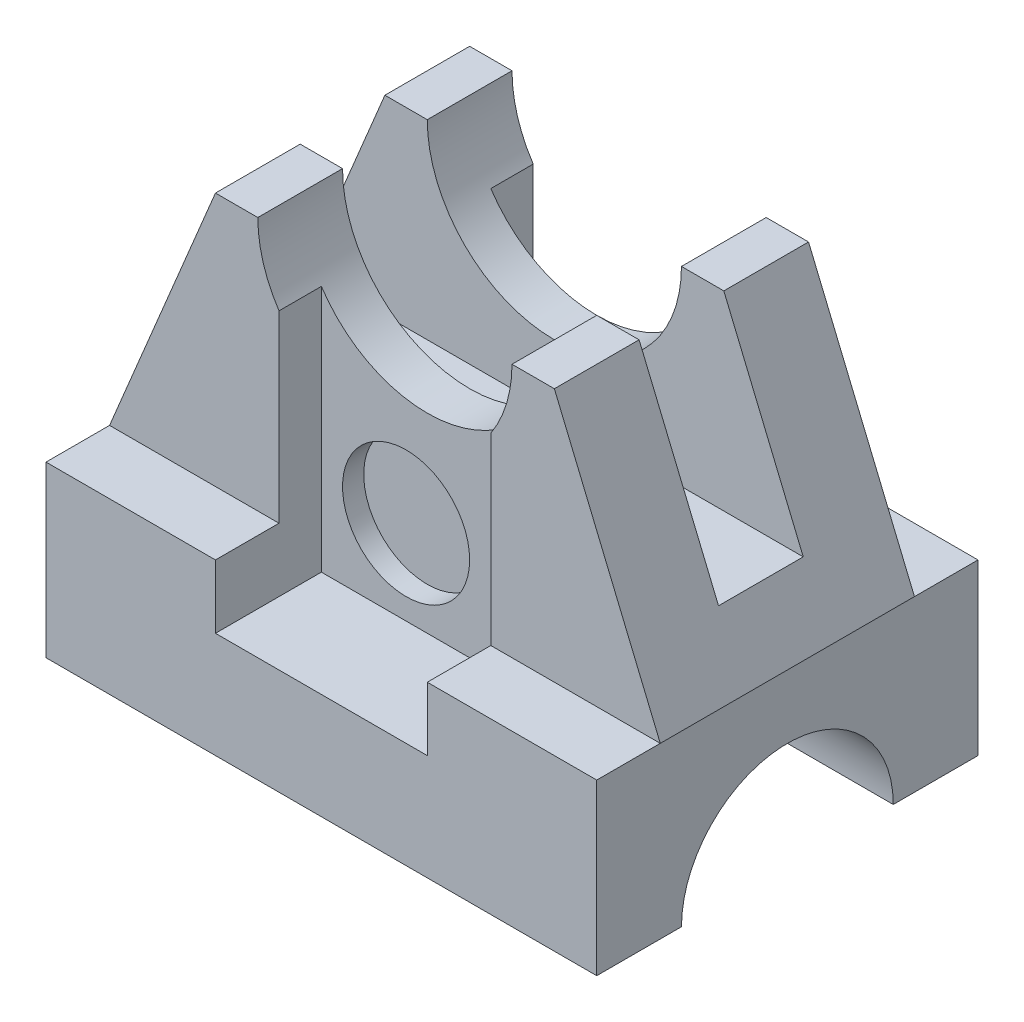
ISO-10303-21;
HEADER;
FILE_DESCRIPTION(('STEP AP214'),'2;1');
FILE_NAME('part.step','',(''),(''),'','','');
FILE_SCHEMA(('AUTOMOTIVE_DESIGN { 1 0 10303 214 1 1 1 1 }'));
ENDSEC;
DATA;
#1=APPLICATION_CONTEXT('core data for automotive mechanical design processes');
#2=APPLICATION_PROTOCOL_DEFINITION('international standard','automotive_design',2000,#1);
#3=PRODUCT_CONTEXT('',#1,'mechanical');
#4=PRODUCT('Part','Part','',(#3));
#5=PRODUCT_RELATED_PRODUCT_CATEGORY('part','',(#4));
#6=PRODUCT_DEFINITION_FORMATION('','',#4);
#7=PRODUCT_DEFINITION_CONTEXT('part definition',#1,'design');
#8=PRODUCT_DEFINITION('design','',#6,#7);
#9=PRODUCT_DEFINITION_SHAPE('','',#8);
#10=(LENGTH_UNIT() NAMED_UNIT(*) SI_UNIT(.MILLI.,.METRE.));
#11=(NAMED_UNIT(*) PLANE_ANGLE_UNIT() SI_UNIT($,.RADIAN.));
#12=(NAMED_UNIT(*) SI_UNIT($,.STERADIAN.) SOLID_ANGLE_UNIT());
#13=UNCERTAINTY_MEASURE_WITH_UNIT(LENGTH_MEASURE(1.E-05),#10,'distance_accuracy_value','');
#14=(GEOMETRIC_REPRESENTATION_CONTEXT(3) GLOBAL_UNCERTAINTY_ASSIGNED_CONTEXT((#13)) GLOBAL_UNIT_ASSIGNED_CONTEXT((#10,
#11,#12)) REPRESENTATION_CONTEXT('',''));
#15=CARTESIAN_POINT('',(0.,0.,0.));
#16=DIRECTION('',(0.,0.,1.));
#17=DIRECTION('',(1.,0.,0.));
#18=AXIS2_PLACEMENT_3D('',#15,#16,#17);
#19=CARTESIAN_POINT('',(0.,0.,-30.));
#20=DIRECTION('',(0.,0.,-1.));
#21=DIRECTION('',(-1.,0.,0.));
#22=AXIS2_PLACEMENT_3D('',#19,#20,#21);
#23=PLANE('',#22);
#24=DIRECTION('',(0.,-1.,0.));
#25=VECTOR('',#24,1.);
#26=CARTESIAN_POINT('',(25.,0.,-30.));
#27=LINE('',#26,#25);
#28=CARTESIAN_POINT('',(25.,58.416876048223,-30.));
#29=VERTEX_POINT('',#28);
#30=CARTESIAN_POINT('',(25.,15.,-30.));
#31=VERTEX_POINT('',#30);
#32=EDGE_CURVE('E261',#29,#31,#27,.T.);
#33=ORIENTED_EDGE('',*,*,#32,.F.);
#34=CARTESIAN_POINT('',(0.,75.,-30.));
#35=DIRECTION('',(0.,0.,-1.));
#36=DIRECTION('',(-1.,0.,0.));
#37=AXIS2_PLACEMENT_3D('',#34,#35,#36);
#38=CIRCLE('',#37,30.);
#39=CARTESIAN_POINT('',(30.,75.,-30.));
#40=VERTEX_POINT('',#39);
#41=EDGE_CURVE('E308',#40,#29,#38,.T.);
#42=ORIENTED_EDGE('',*,*,#41,.F.);
#43=DIRECTION('',(-1.,0.,0.));
#44=VECTOR('',#43,1.);
#45=CARTESIAN_POINT('',(-40.,75.,-30.));
#46=LINE('',#45,#44);
#47=CARTESIAN_POINT('',(40.,75.,-30.));
#48=VERTEX_POINT('',#47);
#49=EDGE_CURVE('E377',#48,#40,#46,.T.);
#50=ORIENTED_EDGE('',*,*,#49,.F.);
#51=DIRECTION('',(-0.384615384615385,0.923076923076923,0.));
#52=VECTOR('',#51,1.);
#53=CARTESIAN_POINT('',(40.,75.,-30.));
#54=LINE('',#53,#52);
#55=CARTESIAN_POINT('',(65.,15.,-30.));
#56=VERTEX_POINT('',#55);
#57=EDGE_CURVE('E372',#56,#48,#54,.T.);
#58=ORIENTED_EDGE('',*,*,#57,.F.);
#59=DIRECTION('',(1.,0.,0.));
#60=VECTOR('',#59,1.);
#61=CARTESIAN_POINT('',(25.,15.,-30.));
#62=LINE('',#61,#60);
#63=EDGE_CURVE('E371',#31,#56,#62,.T.);
#64=ORIENTED_EDGE('',*,*,#63,.F.);
#65=EDGE_LOOP('',(#33,#42,#50,#58,#64));
#66=FACE_BOUND('',#65,.T.);
#67=ADVANCED_FACE('F39',(#66),#23,.T.);
#68=CARTESIAN_POINT('',(0.,0.,30.));
#69=DIRECTION('',(0.,0.,1.));
#70=DIRECTION('',(1.,0.,0.));
#71=AXIS2_PLACEMENT_3D('',#68,#69,#70);
#72=PLANE('',#71);
#73=DIRECTION('',(0.,-1.,0.));
#74=VECTOR('',#73,1.);
#75=CARTESIAN_POINT('',(-25.,0.,30.));
#76=LINE('',#75,#74);
#77=CARTESIAN_POINT('',(-25.,58.416876048223,30.));
#78=VERTEX_POINT('',#77);
#79=CARTESIAN_POINT('',(-25.,15.,30.));
#80=VERTEX_POINT('',#79);
#81=EDGE_CURVE('E278',#78,#80,#76,.T.);
#82=ORIENTED_EDGE('',*,*,#81,.F.);
#83=CARTESIAN_POINT('',(0.,75.,30.));
#84=DIRECTION('',(0.,0.,1.));
#85=DIRECTION('',(1.,0.,0.));
#86=AXIS2_PLACEMENT_3D('',#83,#84,#85);
#87=CIRCLE('',#86,30.);
#88=CARTESIAN_POINT('',(-30.,75.,30.));
#89=VERTEX_POINT('',#88);
#90=EDGE_CURVE('E302',#89,#78,#87,.T.);
#91=ORIENTED_EDGE('',*,*,#90,.F.);
#92=DIRECTION('',(-1.,0.,0.));
#93=VECTOR('',#92,1.);
#94=CARTESIAN_POINT('',(40.,75.,30.));
#95=LINE('',#94,#93);
#96=CARTESIAN_POINT('',(-40.,75.,30.));
#97=VERTEX_POINT('',#96);
#98=EDGE_CURVE('E343',#89,#97,#95,.T.);
#99=ORIENTED_EDGE('',*,*,#98,.T.);
#100=DIRECTION('',(-0.384615384615385,-0.923076923076923,0.));
#101=VECTOR('',#100,1.);
#102=CARTESIAN_POINT('',(-40.,75.,30.));
#103=LINE('',#102,#101);
#104=CARTESIAN_POINT('',(-65.,15.,30.));
#105=VERTEX_POINT('',#104);
#106=EDGE_CURVE('E334',#97,#105,#103,.T.);
#107=ORIENTED_EDGE('',*,*,#106,.T.);
#108=DIRECTION('',(1.,0.,0.));
#109=VECTOR('',#108,1.);
#110=CARTESIAN_POINT('',(-65.,15.,30.));
#111=LINE('',#110,#109);
#112=EDGE_CURVE('E331',#105,#80,#111,.T.);
#113=ORIENTED_EDGE('',*,*,#112,.T.);
#114=EDGE_LOOP('',(#82,#91,#99,#107,#113));
#115=FACE_BOUND('',#114,.T.);
#116=ADVANCED_FACE('F511',(#115),#72,.T.);
#117=CARTESIAN_POINT('',(-40.,75.,-30.));
#118=DIRECTION('',(0.,1.,0.));
#119=DIRECTION('',(0.,0.,1.));
#120=AXIS2_PLACEMENT_3D('',#117,#118,#119);
#121=PLANE('',#120);
#122=DIRECTION('',(0.,0.,-1.));
#123=VECTOR('',#122,1.);
#124=CARTESIAN_POINT('',(30.,75.,45.));
#125=LINE('',#124,#123);
#126=CARTESIAN_POINT('',(30.,75.,30.));
#127=VERTEX_POINT('',#126);
#128=CARTESIAN_POINT('',(30.,75.,10.));
#129=VERTEX_POINT('',#128);
#130=EDGE_CURVE('E298',#127,#129,#125,.T.);
#131=ORIENTED_EDGE('',*,*,#130,.F.);
#132=CARTESIAN_POINT('',(40.,75.,30.));
#133=VERTEX_POINT('',#132);
#134=EDGE_CURVE('E342',#133,#127,#95,.T.);
#135=ORIENTED_EDGE('',*,*,#134,.F.);
#136=DIRECTION('',(0.,0.,1.));
#137=VECTOR('',#136,1.);
#138=CARTESIAN_POINT('',(40.,75.,-30.));
#139=LINE('',#138,#137);
#140=CARTESIAN_POINT('',(40.,75.,10.));
#141=VERTEX_POINT('',#140);
#142=EDGE_CURVE('E381',#141,#133,#139,.T.);
#143=ORIENTED_EDGE('',*,*,#142,.F.);
#144=DIRECTION('',(1.,0.,0.));
#145=VECTOR('',#144,1.);
#146=CARTESIAN_POINT('',(-65.,75.,10.));
#147=LINE('',#146,#145);
#148=EDGE_CURVE('E321',#129,#141,#147,.T.);
#149=ORIENTED_EDGE('',*,*,#148,.F.);
#150=EDGE_LOOP('',(#131,#135,#143,#149));
#151=FACE_BOUND('',#150,.T.);
#152=ADVANCED_FACE('F528',(#151),#121,.T.);
#153=CARTESIAN_POINT('',(30.,75.,-10.));
#154=VERTEX_POINT('',#153);
#155=EDGE_CURVE('E295',#154,#40,#125,.T.);
#156=ORIENTED_EDGE('',*,*,#155,.F.);
#157=DIRECTION('',(-1.,0.,0.));
#158=VECTOR('',#157,1.);
#159=CARTESIAN_POINT('',(-65.,75.,-10.));
#160=LINE('',#159,#158);
#161=CARTESIAN_POINT('',(40.,75.,-10.));
#162=VERTEX_POINT('',#161);
#163=EDGE_CURVE('E316',#162,#154,#160,.T.);
#164=ORIENTED_EDGE('',*,*,#163,.F.);
#165=EDGE_CURVE('E387',#48,#162,#139,.T.);
#166=ORIENTED_EDGE('',*,*,#165,.F.);
#167=ORIENTED_EDGE('',*,*,#49,.T.);
#168=EDGE_LOOP('',(#156,#164,#166,#167));
#169=FACE_BOUND('',#168,.T.);
#170=ADVANCED_FACE('F562',(#169),#121,.T.);
#171=DIRECTION('',(0.,0.,-1.));
#172=VECTOR('',#171,1.);
#173=CARTESIAN_POINT('',(-30.,75.,45.));
#174=LINE('',#173,#172);
#175=CARTESIAN_POINT('',(-30.,75.,10.));
#176=VERTEX_POINT('',#175);
#177=EDGE_CURVE('E300',#89,#176,#174,.T.);
#178=ORIENTED_EDGE('',*,*,#177,.T.);
#179=CARTESIAN_POINT('',(-40.,75.,10.));
#180=VERTEX_POINT('',#179);
#181=EDGE_CURVE('E317',#180,#176,#147,.T.);
#182=ORIENTED_EDGE('',*,*,#181,.F.);
#183=DIRECTION('',(0.,0.,1.));
#184=VECTOR('',#183,1.);
#185=CARTESIAN_POINT('',(-40.,75.,-30.));
#186=LINE('',#185,#184);
#187=EDGE_CURVE('E388',#180,#97,#186,.T.);
#188=ORIENTED_EDGE('',*,*,#187,.T.);
#189=ORIENTED_EDGE('',*,*,#98,.F.);
#190=EDGE_LOOP('',(#178,#182,#188,#189));
#191=FACE_BOUND('',#190,.T.);
#192=ADVANCED_FACE('F525',(#191),#121,.T.);
#193=CARTESIAN_POINT('',(-65.,15.,-30.));
#194=DIRECTION('',(-0.923076923076923,0.384615384615385,0.));
#195=DIRECTION('',(-0.384615384615385,-0.923076923076923,0.));
#196=AXIS2_PLACEMENT_3D('',#193,#194,#195);
#197=PLANE('',#196);
#198=DIRECTION('',(0.384615384615385,0.923076923076923,0.));
#199=VECTOR('',#198,1.);
#200=CARTESIAN_POINT('',(-65.,15.,10.));
#201=LINE('',#200,#199);
#202=CARTESIAN_POINT('',(-58.75,30.,10.));
#203=VERTEX_POINT('',#202);
#204=EDGE_CURVE('E327',#203,#180,#201,.T.);
#205=ORIENTED_EDGE('',*,*,#204,.F.);
#206=DIRECTION('',(0.,0.,-1.));
#207=VECTOR('',#206,1.);
#208=CARTESIAN_POINT('',(-58.75,30.,-30.));
#209=LINE('',#208,#207);
#210=CARTESIAN_POINT('',(-58.75,30.,-10.));
#211=VERTEX_POINT('',#210);
#212=EDGE_CURVE('E319',#203,#211,#209,.T.);
#213=ORIENTED_EDGE('',*,*,#212,.T.);
#214=DIRECTION('',(-0.384615384615385,-0.923076923076923,0.));
#215=VECTOR('',#214,1.);
#216=CARTESIAN_POINT('',(-65.,15.,-10.));
#217=LINE('',#216,#215);
#218=CARTESIAN_POINT('',(-40.,75.,-10.));
#219=VERTEX_POINT('',#218);
#220=EDGE_CURVE('E330',#219,#211,#217,.T.);
#221=ORIENTED_EDGE('',*,*,#220,.F.);
#222=CARTESIAN_POINT('',(-40.,75.,-30.));
#223=VERTEX_POINT('',#222);
#224=EDGE_CURVE('E383',#223,#219,#186,.T.);
#225=ORIENTED_EDGE('',*,*,#224,.F.);
#226=DIRECTION('',(-0.384615384615385,-0.923076923076923,0.));
#227=VECTOR('',#226,1.);
#228=CARTESIAN_POINT('',(-65.,15.,-30.));
#229=LINE('',#228,#227);
#230=CARTESIAN_POINT('',(-65.,15.,-30.));
#231=VERTEX_POINT('',#230);
#232=EDGE_CURVE('E382',#223,#231,#229,.T.);
#233=ORIENTED_EDGE('',*,*,#232,.T.);
#234=DIRECTION('',(0.,0.,-1.));
#235=VECTOR('',#234,1.);
#236=CARTESIAN_POINT('',(-65.,15.,45.));
#237=LINE('',#236,#235);
#238=EDGE_CURVE('E446',#105,#231,#237,.T.);
#239=ORIENTED_EDGE('',*,*,#238,.F.);
#240=ORIENTED_EDGE('',*,*,#106,.F.);
#241=ORIENTED_EDGE('',*,*,#187,.F.);
#242=EDGE_LOOP('',(#205,#213,#221,#225,#233,#239,#240,#241));
#243=FACE_BOUND('',#242,.T.);
#244=ADVANCED_FACE('F480',(#243),#197,.T.);
#245=CARTESIAN_POINT('',(-30.,75.,-10.));
#246=VERTEX_POINT('',#245);
#247=CARTESIAN_POINT('',(-30.,75.,-30.));
#248=VERTEX_POINT('',#247);
#249=EDGE_CURVE('E293',#246,#248,#174,.T.);
#250=ORIENTED_EDGE('',*,*,#249,.T.);
#251=EDGE_CURVE('E380',#248,#223,#46,.T.);
#252=ORIENTED_EDGE('',*,*,#251,.T.);
#253=ORIENTED_EDGE('',*,*,#224,.T.);
#254=EDGE_CURVE('E311',#246,#219,#160,.T.);
#255=ORIENTED_EDGE('',*,*,#254,.F.);
#256=EDGE_LOOP('',(#250,#252,#253,#255));
#257=FACE_BOUND('',#256,.T.);
#258=ADVANCED_FACE('F479',(#257),#121,.T.);
#259=CARTESIAN_POINT('',(40.,75.,-30.));
#260=DIRECTION('',(0.923076923076923,0.384615384615385,0.));
#261=DIRECTION('',(-0.384615384615385,0.923076923076923,0.));
#262=AXIS2_PLACEMENT_3D('',#259,#260,#261);
#263=PLANE('',#262);
#264=DIRECTION('',(0.384615384615385,-0.923076923076923,0.));
#265=VECTOR('',#264,1.);
#266=CARTESIAN_POINT('',(40.,75.,10.));
#267=LINE('',#266,#265);
#268=CARTESIAN_POINT('',(58.75,30.,9.99999999999999));
#269=VERTEX_POINT('',#268);
#270=EDGE_CURVE('E50',#141,#269,#267,.T.);
#271=ORIENTED_EDGE('',*,*,#270,.F.);
#272=ORIENTED_EDGE('',*,*,#142,.T.);
#273=DIRECTION('',(-0.384615384615385,0.923076923076923,0.));
#274=VECTOR('',#273,1.);
#275=CARTESIAN_POINT('',(65.,15.,30.));
#276=LINE('',#275,#274);
#277=CARTESIAN_POINT('',(65.,15.,30.));
#278=VERTEX_POINT('',#277);
#279=EDGE_CURVE('E344',#278,#133,#276,.T.);
#280=ORIENTED_EDGE('',*,*,#279,.F.);
#281=DIRECTION('',(0.,0.,-1.));
#282=VECTOR('',#281,1.);
#283=CARTESIAN_POINT('',(65.,15.,45.));
#284=LINE('',#283,#282);
#285=EDGE_CURVE('E440',#278,#56,#284,.T.);
#286=ORIENTED_EDGE('',*,*,#285,.T.);
#287=ORIENTED_EDGE('',*,*,#57,.T.);
#288=ORIENTED_EDGE('',*,*,#165,.T.);
#289=DIRECTION('',(-0.384615384615385,0.923076923076923,0.));
#290=VECTOR('',#289,1.);
#291=CARTESIAN_POINT('',(40.,75.,-10.));
#292=LINE('',#291,#290);
#293=CARTESIAN_POINT('',(58.75,30.,-10.));
#294=VERTEX_POINT('',#293);
#295=EDGE_CURVE('E452',#294,#162,#292,.T.);
#296=ORIENTED_EDGE('',*,*,#295,.F.);
#297=DIRECTION('',(0.,0.,1.));
#298=VECTOR('',#297,1.);
#299=CARTESIAN_POINT('',(58.75,30.,-30.));
#300=LINE('',#299,#298);
#301=EDGE_CURVE('E451',#294,#269,#300,.T.);
#302=ORIENTED_EDGE('',*,*,#301,.T.);
#303=EDGE_LOOP('',(#271,#272,#280,#286,#287,#288,#296,#302));
#304=FACE_BOUND('',#303,.T.);
#305=ADVANCED_FACE('F467',(#304),#263,.T.);
#306=CARTESIAN_POINT('',(-25.,15.,45.));
#307=DIRECTION('',(-1.,0.,0.));
#308=DIRECTION('',(0.,0.,1.));
#309=AXIS2_PLACEMENT_3D('',#306,#307,#308);
#310=PLANE('',#309);
#311=DIRECTION('',(0.,0.,-1.));
#312=VECTOR('',#311,1.);
#313=CARTESIAN_POINT('',(-25.,15.,45.));
#314=LINE('',#313,#312);
#315=CARTESIAN_POINT('',(-25.,15.,-30.));
#316=VERTEX_POINT('',#315);
#317=CARTESIAN_POINT('',(-25.,15.,-45.));
#318=VERTEX_POINT('',#317);
#319=EDGE_CURVE('E449',#316,#318,#314,.T.);
#320=ORIENTED_EDGE('',*,*,#319,.F.);
#321=DIRECTION('',(0.,1.,0.));
#322=VECTOR('',#321,1.);
#323=CARTESIAN_POINT('',(-25.,0.,-30.));
#324=LINE('',#323,#322);
#325=CARTESIAN_POINT('',(-25.,58.416876048223,-30.));
#326=VERTEX_POINT('',#325);
#327=EDGE_CURVE('E258',#316,#326,#324,.T.);
#328=ORIENTED_EDGE('',*,*,#327,.T.);
#329=DIRECTION('',(0.,0.,-1.));
#330=VECTOR('',#329,1.);
#331=CARTESIAN_POINT('',(-25.,58.416876048223,-20.));
#332=LINE('',#331,#330);
#333=CARTESIAN_POINT('',(-25.,58.416876048223,-20.));
#334=VERTEX_POINT('',#333);
#335=EDGE_CURVE('E270',#334,#326,#332,.T.);
#336=ORIENTED_EDGE('',*,*,#335,.F.);
#337=DIRECTION('',(0.,1.,0.));
#338=VECTOR('',#337,1.);
#339=CARTESIAN_POINT('',(-25.,0.,-20.));
#340=LINE('',#339,#338);
#341=CARTESIAN_POINT('',(-25.,0.,-20.));
#342=VERTEX_POINT('',#341);
#343=EDGE_CURVE('E53',#342,#334,#340,.T.);
#344=ORIENTED_EDGE('',*,*,#343,.F.);
#345=DIRECTION('',(0.,0.,-1.));
#346=VECTOR('',#345,1.);
#347=CARTESIAN_POINT('',(-25.,0.,45.));
#348=LINE('',#347,#346);
#349=CARTESIAN_POINT('',(-25.,0.,-45.));
#350=VERTEX_POINT('',#349);
#351=EDGE_CURVE('E254',#342,#350,#348,.T.);
#352=ORIENTED_EDGE('',*,*,#351,.T.);
#353=DIRECTION('',(0.,1.,0.));
#354=VECTOR('',#353,1.);
#355=CARTESIAN_POINT('',(-25.,15.,-45.));
#356=LINE('',#355,#354);
#357=EDGE_CURVE('E401',#350,#318,#356,.T.);
#358=ORIENTED_EDGE('',*,*,#357,.T.);
#359=EDGE_LOOP('',(#320,#328,#336,#344,#352,#358));
#360=FACE_BOUND('',#359,.T.);
#361=ADVANCED_FACE('F41',(#360),#310,.F.);
#362=CARTESIAN_POINT('',(-65.,15.,45.));
#363=DIRECTION('',(0.,-1.,0.));
#364=DIRECTION('',(0.,0.,-1.));
#365=AXIS2_PLACEMENT_3D('',#362,#363,#364);
#366=PLANE('',#365);
#367=CARTESIAN_POINT('',(-65.,15.,-45.));
#368=VERTEX_POINT('',#367);
#369=EDGE_CURVE('E443',#231,#368,#237,.T.);
#370=ORIENTED_EDGE('',*,*,#369,.F.);
#371=DIRECTION('',(1.,0.,0.));
#372=VECTOR('',#371,1.);
#373=CARTESIAN_POINT('',(-65.,15.,-30.));
#374=LINE('',#373,#372);
#375=EDGE_CURVE('E361',#231,#316,#374,.T.);
#376=ORIENTED_EDGE('',*,*,#375,.T.);
#377=ORIENTED_EDGE('',*,*,#319,.T.);
#378=DIRECTION('',(-1.,0.,0.));
#379=VECTOR('',#378,1.);
#380=CARTESIAN_POINT('',(-65.,15.,-45.));
#381=LINE('',#380,#379);
#382=EDGE_CURVE('E414',#318,#368,#381,.T.);
#383=ORIENTED_EDGE('',*,*,#382,.T.);
#384=EDGE_LOOP('',(#370,#376,#377,#383));
#385=FACE_BOUND('',#384,.T.);
#386=ADVANCED_FACE('F489',(#385),#366,.F.);
#387=CARTESIAN_POINT('',(-65.,-25.,45.));
#388=DIRECTION('',(1.,0.,0.));
#389=DIRECTION('',(0.,0.,-1.));
#390=AXIS2_PLACEMENT_3D('',#387,#388,#389);
#391=PLANE('',#390);
#392=DIRECTION('',(0.,-1.,0.));
#393=VECTOR('',#392,1.);
#394=CARTESIAN_POINT('',(-65.,-25.,-45.));
#395=LINE('',#394,#393);
#396=CARTESIAN_POINT('',(-65.,-25.,-45.));
#397=VERTEX_POINT('',#396);
#398=EDGE_CURVE('E417',#368,#397,#395,.T.);
#399=ORIENTED_EDGE('',*,*,#398,.T.);
#400=DIRECTION('',(0.,0.,-1.));
#401=VECTOR('',#400,1.);
#402=CARTESIAN_POINT('',(-65.,-25.,45.));
#403=LINE('',#402,#401);
#404=CARTESIAN_POINT('',(-65.,-25.,45.));
#405=VERTEX_POINT('',#404);
#406=EDGE_CURVE('E441',#405,#397,#403,.T.);
#407=ORIENTED_EDGE('',*,*,#406,.F.);
#408=DIRECTION('',(0.,-1.,0.));
#409=VECTOR('',#408,1.);
#410=CARTESIAN_POINT('',(-65.,-25.,45.));
#411=LINE('',#410,#409);
#412=CARTESIAN_POINT('',(-65.,15.,45.));
#413=VERTEX_POINT('',#412);
#414=EDGE_CURVE('E409',#413,#405,#411,.T.);
#415=ORIENTED_EDGE('',*,*,#414,.F.);
#416=EDGE_CURVE('E444',#413,#105,#237,.T.);
#417=ORIENTED_EDGE('',*,*,#416,.T.);
#418=ORIENTED_EDGE('',*,*,#238,.T.);
#419=ORIENTED_EDGE('',*,*,#369,.T.);
#420=EDGE_LOOP('',(#399,#407,#415,#417,#418,#419));
#421=FACE_BOUND('',#420,.T.);
#422=ADVANCED_FACE('F492',(#421),#391,.F.);
#423=CARTESIAN_POINT('',(65.,-25.,45.));
#424=DIRECTION('',(0.,1.,0.));
#425=DIRECTION('',(-1.,0.,0.));
#426=AXIS2_PLACEMENT_3D('',#423,#424,#425);
#427=PLANE('',#426);
#428=DIRECTION('',(0.,0.,-1.));
#429=VECTOR('',#428,1.);
#430=CARTESIAN_POINT('',(35.,-25.,25.));
#431=LINE('',#430,#429);
#432=CARTESIAN_POINT('',(35.,-25.,25.));
#433=VERTEX_POINT('',#432);
#434=CARTESIAN_POINT('',(35.,-25.,-25.));
#435=VERTEX_POINT('',#434);
#436=EDGE_CURVE('E398',#433,#435,#431,.T.);
#437=ORIENTED_EDGE('',*,*,#436,.F.);
#438=DIRECTION('',(1.,0.,0.));
#439=VECTOR('',#438,1.);
#440=CARTESIAN_POINT('',(35.,-25.,25.));
#441=LINE('',#440,#439);
#442=CARTESIAN_POINT('',(65.,-25.,25.));
#443=VERTEX_POINT('',#442);
#444=EDGE_CURVE('E400',#433,#443,#441,.T.);
#445=ORIENTED_EDGE('',*,*,#444,.T.);
#446=DIRECTION('',(0.,0.,-1.));
#447=VECTOR('',#446,1.);
#448=CARTESIAN_POINT('',(65.,-25.,45.));
#449=LINE('',#448,#447);
#450=CARTESIAN_POINT('',(65.,-25.,45.));
#451=VERTEX_POINT('',#450);
#452=EDGE_CURVE('E438',#451,#443,#449,.T.);
#453=ORIENTED_EDGE('',*,*,#452,.F.);
#454=DIRECTION('',(1.,0.,0.));
#455=VECTOR('',#454,1.);
#456=CARTESIAN_POINT('',(65.,-25.,45.));
#457=LINE('',#456,#455);
#458=EDGE_CURVE('E410',#405,#451,#457,.T.);
#459=ORIENTED_EDGE('',*,*,#458,.F.);
#460=ORIENTED_EDGE('',*,*,#406,.T.);
#461=DIRECTION('',(1.,0.,0.));
#462=VECTOR('',#461,1.);
#463=CARTESIAN_POINT('',(65.,-25.,-45.));
#464=LINE('',#463,#462);
#465=CARTESIAN_POINT('',(65.,-25.,-45.));
#466=VERTEX_POINT('',#465);
#467=EDGE_CURVE('E416',#397,#466,#464,.T.);
#468=ORIENTED_EDGE('',*,*,#467,.T.);
#469=CARTESIAN_POINT('',(65.,-25.,-25.));
#470=VERTEX_POINT('',#469);
#471=EDGE_CURVE('E436',#470,#466,#449,.T.);
#472=ORIENTED_EDGE('',*,*,#471,.F.);
#473=DIRECTION('',(1.,0.,0.));
#474=VECTOR('',#473,1.);
#475=CARTESIAN_POINT('',(35.,-25.,-25.));
#476=LINE('',#475,#474);
#477=EDGE_CURVE('E402',#435,#470,#476,.T.);
#478=ORIENTED_EDGE('',*,*,#477,.F.);
#479=EDGE_LOOP('',(#437,#445,#453,#459,#460,#468,#472,#478));
#480=FACE_BOUND('',#479,.T.);
#481=ADVANCED_FACE('F612',(#480),#427,.F.);
#482=CARTESIAN_POINT('',(65.,15.,45.));
#483=DIRECTION('',(-1.,0.,0.));
#484=DIRECTION('',(0.,0.,1.));
#485=AXIS2_PLACEMENT_3D('',#482,#483,#484);
#486=PLANE('',#485);
#487=ORIENTED_EDGE('',*,*,#452,.T.);
#488=CARTESIAN_POINT('',(65.,-25.,0.));
#489=DIRECTION('',(1.,0.,0.));
#490=DIRECTION('',(0.,0.,-1.));
#491=AXIS2_PLACEMENT_3D('',#488,#489,#490);
#492=CIRCLE('',#491,25.);
#493=EDGE_CURVE('E390',#470,#443,#492,.T.);
#494=ORIENTED_EDGE('',*,*,#493,.F.);
#495=ORIENTED_EDGE('',*,*,#471,.T.);
#496=DIRECTION('',(0.,1.,0.));
#497=VECTOR('',#496,1.);
#498=CARTESIAN_POINT('',(65.,15.,-45.));
#499=LINE('',#498,#497);
#500=CARTESIAN_POINT('',(65.,15.,-45.));
#501=VERTEX_POINT('',#500);
#502=EDGE_CURVE('E421',#466,#501,#499,.T.);
#503=ORIENTED_EDGE('',*,*,#502,.T.);
#504=EDGE_CURVE('E435',#56,#501,#284,.T.);
#505=ORIENTED_EDGE('',*,*,#504,.F.);
#506=ORIENTED_EDGE('',*,*,#285,.F.);
#507=CARTESIAN_POINT('',(65.,15.,45.));
#508=VERTEX_POINT('',#507);
#509=EDGE_CURVE('E433',#508,#278,#284,.T.);
#510=ORIENTED_EDGE('',*,*,#509,.F.);
#511=DIRECTION('',(0.,1.,0.));
#512=VECTOR('',#511,1.);
#513=CARTESIAN_POINT('',(65.,15.,45.));
#514=LINE('',#513,#512);
#515=EDGE_CURVE('E248',#451,#508,#514,.T.);
#516=ORIENTED_EDGE('',*,*,#515,.F.);
#517=EDGE_LOOP('',(#487,#494,#495,#503,#505,#506,#510,#516));
#518=FACE_BOUND('',#517,.T.);
#519=ADVANCED_FACE('F537',(#518),#486,.F.);
#520=CARTESIAN_POINT('',(25.,15.,45.));
#521=DIRECTION('',(0.,-1.,0.));
#522=DIRECTION('',(0.,0.,-1.));
#523=AXIS2_PLACEMENT_3D('',#520,#521,#522);
#524=PLANE('',#523);
#525=DIRECTION('',(0.,0.,-1.));
#526=VECTOR('',#525,1.);
#527=CARTESIAN_POINT('',(25.,15.,45.));
#528=LINE('',#527,#526);
#529=CARTESIAN_POINT('',(25.,15.,-45.));
#530=VERTEX_POINT('',#529);
#531=EDGE_CURVE('E247',#31,#530,#528,.T.);
#532=ORIENTED_EDGE('',*,*,#531,.F.);
#533=ORIENTED_EDGE('',*,*,#63,.T.);
#534=ORIENTED_EDGE('',*,*,#504,.T.);
#535=DIRECTION('',(-1.,0.,0.));
#536=VECTOR('',#535,1.);
#537=CARTESIAN_POINT('',(25.,15.,-45.));
#538=LINE('',#537,#536);
#539=EDGE_CURVE('E428',#501,#530,#538,.T.);
#540=ORIENTED_EDGE('',*,*,#539,.T.);
#541=EDGE_LOOP('',(#532,#533,#534,#540));
#542=FACE_BOUND('',#541,.T.);
#543=ADVANCED_FACE('F544',(#542),#524,.F.);
#544=CARTESIAN_POINT('',(25.,0.,45.));
#545=DIRECTION('',(1.,0.,0.));
#546=DIRECTION('',(0.,0.,-1.));
#547=AXIS2_PLACEMENT_3D('',#544,#545,#546);
#548=PLANE('',#547);
#549=DIRECTION('',(0.,0.,-1.));
#550=VECTOR('',#549,1.);
#551=CARTESIAN_POINT('',(25.,0.,45.));
#552=LINE('',#551,#550);
#553=CARTESIAN_POINT('',(25.,0.,-20.));
#554=VERTEX_POINT('',#553);
#555=CARTESIAN_POINT('',(25.,0.,-45.));
#556=VERTEX_POINT('',#555);
#557=EDGE_CURVE('E238',#554,#556,#552,.T.);
#558=ORIENTED_EDGE('',*,*,#557,.F.);
#559=DIRECTION('',(0.,-1.,0.));
#560=VECTOR('',#559,1.);
#561=CARTESIAN_POINT('',(25.,0.,-20.));
#562=LINE('',#561,#560);
#563=CARTESIAN_POINT('',(25.,58.416876048223,-20.));
#564=VERTEX_POINT('',#563);
#565=EDGE_CURVE('E245',#564,#554,#562,.T.);
#566=ORIENTED_EDGE('',*,*,#565,.F.);
#567=DIRECTION('',(0.,0.,-1.));
#568=VECTOR('',#567,1.);
#569=CARTESIAN_POINT('',(25.,58.416876048223,-20.));
#570=LINE('',#569,#568);
#571=EDGE_CURVE('E275',#564,#29,#570,.T.);
#572=ORIENTED_EDGE('',*,*,#571,.T.);
#573=ORIENTED_EDGE('',*,*,#32,.T.);
#574=ORIENTED_EDGE('',*,*,#531,.T.);
#575=DIRECTION('',(0.,-1.,0.));
#576=VECTOR('',#575,1.);
#577=CARTESIAN_POINT('',(25.,0.,-45.));
#578=LINE('',#577,#576);
#579=EDGE_CURVE('E242',#530,#556,#578,.T.);
#580=ORIENTED_EDGE('',*,*,#579,.T.);
#581=EDGE_LOOP('',(#558,#566,#572,#573,#574,#580));
#582=FACE_BOUND('',#581,.T.);
#583=ADVANCED_FACE('F239',(#582),#548,.F.);
#584=CARTESIAN_POINT('',(0.,0.,45.));
#585=DIRECTION('',(0.,-1.,0.));
#586=DIRECTION('',(0.,0.,-1.));
#587=AXIS2_PLACEMENT_3D('',#584,#585,#586);
#588=PLANE('',#587);
#589=ORIENTED_EDGE('',*,*,#351,.F.);
#590=DIRECTION('',(-1.,0.,0.));
#591=VECTOR('',#590,1.);
#592=CARTESIAN_POINT('',(25.,0.,-20.));
#593=LINE('',#592,#591);
#594=EDGE_CURVE('E252',#554,#342,#593,.T.);
#595=ORIENTED_EDGE('',*,*,#594,.F.);
#596=ORIENTED_EDGE('',*,*,#557,.T.);
#597=DIRECTION('',(-1.,0.,0.));
#598=VECTOR('',#597,1.);
#599=CARTESIAN_POINT('',(0.,0.,-45.));
#600=LINE('',#599,#598);
#601=EDGE_CURVE('E408',#556,#350,#600,.T.);
#602=ORIENTED_EDGE('',*,*,#601,.T.);
#603=EDGE_LOOP('',(#589,#595,#596,#602));
#604=FACE_BOUND('',#603,.T.);
#605=ADVANCED_FACE('F255',(#604),#588,.F.);
#606=CARTESIAN_POINT('',(0.,0.,45.));
#607=DIRECTION('',(0.,0.,1.));
#608=DIRECTION('',(1.,0.,0.));
#609=AXIS2_PLACEMENT_3D('',#606,#607,#608);
#610=PLANE('',#609);
#611=DIRECTION('',(1.,0.,0.));
#612=VECTOR('',#611,1.);
#613=CARTESIAN_POINT('',(25.,15.,45.));
#614=LINE('',#613,#612);
#615=CARTESIAN_POINT('',(25.,15.,45.));
#616=VERTEX_POINT('',#615);
#617=EDGE_CURVE('E337',#616,#508,#614,.T.);
#618=ORIENTED_EDGE('',*,*,#617,.F.);
#619=DIRECTION('',(0.,1.,0.));
#620=VECTOR('',#619,1.);
#621=CARTESIAN_POINT('',(25.,0.,45.));
#622=LINE('',#621,#620);
#623=CARTESIAN_POINT('',(25.,0.,45.));
#624=VERTEX_POINT('',#623);
#625=EDGE_CURVE('E357',#624,#616,#622,.T.);
#626=ORIENTED_EDGE('',*,*,#625,.F.);
#627=DIRECTION('',(1.,0.,0.));
#628=VECTOR('',#627,1.);
#629=CARTESIAN_POINT('',(-25.,0.,45.));
#630=LINE('',#629,#628);
#631=CARTESIAN_POINT('',(-25.,0.,45.));
#632=VERTEX_POINT('',#631);
#633=EDGE_CURVE('E355',#632,#624,#630,.T.);
#634=ORIENTED_EDGE('',*,*,#633,.F.);
#635=DIRECTION('',(0.,-1.,0.));
#636=VECTOR('',#635,1.);
#637=CARTESIAN_POINT('',(-25.,15.,45.));
#638=LINE('',#637,#636);
#639=CARTESIAN_POINT('',(-25.,15.,45.));
#640=VERTEX_POINT('',#639);
#641=EDGE_CURVE('E353',#640,#632,#638,.T.);
#642=ORIENTED_EDGE('',*,*,#641,.F.);
#643=DIRECTION('',(1.,0.,0.));
#644=VECTOR('',#643,1.);
#645=CARTESIAN_POINT('',(-65.,15.,45.));
#646=LINE('',#645,#644);
#647=EDGE_CURVE('E333',#413,#640,#646,.T.);
#648=ORIENTED_EDGE('',*,*,#647,.F.);
#649=ORIENTED_EDGE('',*,*,#414,.T.);
#650=ORIENTED_EDGE('',*,*,#458,.T.);
#651=ORIENTED_EDGE('',*,*,#515,.T.);
#652=EDGE_LOOP('',(#618,#626,#634,#642,#648,#649,#650,#651));
#653=FACE_BOUND('',#652,.T.);
#654=ADVANCED_FACE('F504',(#653),#610,.T.);
#655=CARTESIAN_POINT('',(0.,0.,-45.));
#656=DIRECTION('',(0.,0.,1.));
#657=DIRECTION('',(1.,0.,0.));
#658=AXIS2_PLACEMENT_3D('',#655,#656,#657);
#659=PLANE('',#658);
#660=ORIENTED_EDGE('',*,*,#357,.F.);
#661=ORIENTED_EDGE('',*,*,#601,.F.);
#662=ORIENTED_EDGE('',*,*,#579,.F.);
#663=ORIENTED_EDGE('',*,*,#539,.F.);
#664=ORIENTED_EDGE('',*,*,#502,.F.);
#665=ORIENTED_EDGE('',*,*,#467,.F.);
#666=ORIENTED_EDGE('',*,*,#398,.F.);
#667=ORIENTED_EDGE('',*,*,#382,.F.);
#668=EDGE_LOOP('',(#660,#661,#662,#663,#664,#665,#666,#667));
#669=FACE_BOUND('',#668,.T.);
#670=ADVANCED_FACE('F555',(#669),#659,.F.);
#671=CARTESIAN_POINT('',(35.,-25.,0.));
#672=DIRECTION('',(1.,0.,0.));
#673=DIRECTION('',(0.,0.,-1.));
#674=AXIS2_PLACEMENT_3D('',#671,#672,#673);
#675=CYLINDRICAL_SURFACE('',#674,25.);
#676=ORIENTED_EDGE('',*,*,#493,.T.);
#677=ORIENTED_EDGE('',*,*,#444,.F.);
#678=CARTESIAN_POINT('',(35.,-25.,0.));
#679=DIRECTION('',(1.,0.,0.));
#680=DIRECTION('',(0.,0.,-1.));
#681=AXIS2_PLACEMENT_3D('',#678,#679,#680);
#682=CIRCLE('',#681,25.);
#683=EDGE_CURVE('E393',#435,#433,#682,.T.);
#684=ORIENTED_EDGE('',*,*,#683,.F.);
#685=ORIENTED_EDGE('',*,*,#477,.T.);
#686=EDGE_LOOP('',(#676,#677,#684,#685));
#687=FACE_BOUND('',#686,.T.);
#688=ADVANCED_FACE('F594',(#687),#675,.F.);
#689=CARTESIAN_POINT('',(35.,-25.,0.));
#690=DIRECTION('',(1.,0.,0.));
#691=DIRECTION('',(0.,0.,-1.));
#692=AXIS2_PLACEMENT_3D('',#689,#690,#691);
#693=PLANE('',#692);
#694=ORIENTED_EDGE('',*,*,#683,.T.);
#695=ORIENTED_EDGE('',*,*,#436,.T.);
#696=EDGE_LOOP('',(#694,#695));
#697=FACE_BOUND('',#696,.T.);
#698=ADVANCED_FACE('F585',(#697),#693,.T.);
#699=ORIENTED_EDGE('',*,*,#327,.F.);
#700=ORIENTED_EDGE('',*,*,#375,.F.);
#701=ORIENTED_EDGE('',*,*,#232,.F.);
#702=ORIENTED_EDGE('',*,*,#251,.F.);
#703=EDGE_CURVE('E310',#326,#248,#38,.T.);
#704=ORIENTED_EDGE('',*,*,#703,.F.);
#705=EDGE_LOOP('',(#699,#700,#701,#702,#704));
#706=FACE_BOUND('',#705,.T.);
#707=ADVANCED_FACE('F485',(#706),#23,.T.);
#708=CARTESIAN_POINT('',(25.,15.,30.));
#709=DIRECTION('',(0.,-1.,0.));
#710=DIRECTION('',(1.,0.,0.));
#711=AXIS2_PLACEMENT_3D('',#708,#709,#710);
#712=PLANE('',#711);
#713=ORIENTED_EDGE('',*,*,#617,.T.);
#714=ORIENTED_EDGE('',*,*,#509,.T.);
#715=DIRECTION('',(1.,0.,0.));
#716=VECTOR('',#715,1.);
#717=CARTESIAN_POINT('',(25.,15.,30.));
#718=LINE('',#717,#716);
#719=CARTESIAN_POINT('',(25.,15.,30.));
#720=VERTEX_POINT('',#719);
#721=EDGE_CURVE('E339',#720,#278,#718,.T.);
#722=ORIENTED_EDGE('',*,*,#721,.F.);
#723=DIRECTION('',(0.,0.,1.));
#724=VECTOR('',#723,1.);
#725=CARTESIAN_POINT('',(25.,15.,30.));
#726=LINE('',#725,#724);
#727=EDGE_CURVE('E363',#720,#616,#726,.T.);
#728=ORIENTED_EDGE('',*,*,#727,.T.);
#729=EDGE_LOOP('',(#713,#714,#722,#728));
#730=FACE_BOUND('',#729,.T.);
#731=ADVANCED_FACE('F536',(#730),#712,.F.);
#732=CARTESIAN_POINT('',(25.,0.,30.));
#733=DIRECTION('',(1.,0.,0.));
#734=DIRECTION('',(0.,0.,-1.));
#735=AXIS2_PLACEMENT_3D('',#732,#733,#734);
#736=PLANE('',#735);
#737=ORIENTED_EDGE('',*,*,#625,.T.);
#738=ORIENTED_EDGE('',*,*,#727,.F.);
#739=DIRECTION('',(0.,1.,0.));
#740=VECTOR('',#739,1.);
#741=CARTESIAN_POINT('',(25.,0.,30.));
#742=LINE('',#741,#740);
#743=CARTESIAN_POINT('',(25.,58.416876048223,30.));
#744=VERTEX_POINT('',#743);
#745=EDGE_CURVE('E274',#720,#744,#742,.T.);
#746=ORIENTED_EDGE('',*,*,#745,.T.);
#747=DIRECTION('',(0.,0.,1.));
#748=VECTOR('',#747,1.);
#749=CARTESIAN_POINT('',(25.,58.416876048223,20.));
#750=LINE('',#749,#748);
#751=CARTESIAN_POINT('',(25.,58.416876048223,20.));
#752=VERTEX_POINT('',#751);
#753=EDGE_CURVE('E288',#752,#744,#750,.T.);
#754=ORIENTED_EDGE('',*,*,#753,.F.);
#755=DIRECTION('',(0.,1.,0.));
#756=VECTOR('',#755,1.);
#757=CARTESIAN_POINT('',(25.,0.,20.));
#758=LINE('',#757,#756);
#759=CARTESIAN_POINT('',(25.,0.,20.));
#760=VERTEX_POINT('',#759);
#761=EDGE_CURVE('E61',#760,#752,#758,.T.);
#762=ORIENTED_EDGE('',*,*,#761,.F.);
#763=DIRECTION('',(0.,0.,1.));
#764=VECTOR('',#763,1.);
#765=CARTESIAN_POINT('',(25.,0.,30.));
#766=LINE('',#765,#764);
#767=EDGE_CURVE('E364',#760,#624,#766,.T.);
#768=ORIENTED_EDGE('',*,*,#767,.T.);
#769=EDGE_LOOP('',(#737,#738,#746,#754,#762,#768));
#770=FACE_BOUND('',#769,.T.);
#771=ADVANCED_FACE('F587',(#770),#736,.F.);
#772=CARTESIAN_POINT('',(-25.,0.,30.));
#773=DIRECTION('',(0.,-1.,0.));
#774=DIRECTION('',(0.,0.,-1.));
#775=AXIS2_PLACEMENT_3D('',#772,#773,#774);
#776=PLANE('',#775);
#777=ORIENTED_EDGE('',*,*,#633,.T.);
#778=ORIENTED_EDGE('',*,*,#767,.F.);
#779=DIRECTION('',(1.,0.,0.));
#780=VECTOR('',#779,1.);
#781=CARTESIAN_POINT('',(-25.,0.,20.));
#782=LINE('',#781,#780);
#783=CARTESIAN_POINT('',(-25.,0.,20.));
#784=VERTEX_POINT('',#783);
#785=EDGE_CURVE('E276',#784,#760,#782,.T.);
#786=ORIENTED_EDGE('',*,*,#785,.F.);
#787=DIRECTION('',(0.,0.,1.));
#788=VECTOR('',#787,1.);
#789=CARTESIAN_POINT('',(-25.,0.,30.));
#790=LINE('',#789,#788);
#791=EDGE_CURVE('E366',#784,#632,#790,.T.);
#792=ORIENTED_EDGE('',*,*,#791,.T.);
#793=EDGE_LOOP('',(#777,#778,#786,#792));
#794=FACE_BOUND('',#793,.T.);
#795=ADVANCED_FACE('F703',(#794),#776,.F.);
#796=CARTESIAN_POINT('',(-25.,15.,30.));
#797=DIRECTION('',(-1.,0.,0.));
#798=DIRECTION('',(0.,-1.,0.));
#799=AXIS2_PLACEMENT_3D('',#796,#797,#798);
#800=PLANE('',#799);
#801=ORIENTED_EDGE('',*,*,#641,.T.);
#802=ORIENTED_EDGE('',*,*,#791,.F.);
#803=DIRECTION('',(0.,-1.,0.));
#804=VECTOR('',#803,1.);
#805=CARTESIAN_POINT('',(-25.,0.,20.));
#806=LINE('',#805,#804);
#807=CARTESIAN_POINT('',(-25.,58.416876048223,20.));
#808=VERTEX_POINT('',#807);
#809=EDGE_CURVE('E283',#808,#784,#806,.T.);
#810=ORIENTED_EDGE('',*,*,#809,.F.);
#811=DIRECTION('',(0.,0.,1.));
#812=VECTOR('',#811,1.);
#813=CARTESIAN_POINT('',(-25.,58.416876048223,20.));
#814=LINE('',#813,#812);
#815=EDGE_CURVE('E290',#808,#78,#814,.T.);
#816=ORIENTED_EDGE('',*,*,#815,.T.);
#817=ORIENTED_EDGE('',*,*,#81,.T.);
#818=DIRECTION('',(0.,0.,1.));
#819=VECTOR('',#818,1.);
#820=CARTESIAN_POINT('',(-25.,15.,30.));
#821=LINE('',#820,#819);
#822=EDGE_CURVE('E348',#80,#640,#821,.T.);
#823=ORIENTED_EDGE('',*,*,#822,.T.);
#824=EDGE_LOOP('',(#801,#802,#810,#816,#817,#823));
#825=FACE_BOUND('',#824,.T.);
#826=ADVANCED_FACE('F508',(#825),#800,.F.);
#827=CARTESIAN_POINT('',(-65.,15.,30.));
#828=DIRECTION('',(0.,-1.,0.));
#829=DIRECTION('',(1.,0.,0.));
#830=AXIS2_PLACEMENT_3D('',#827,#828,#829);
#831=PLANE('',#830);
#832=ORIENTED_EDGE('',*,*,#647,.T.);
#833=ORIENTED_EDGE('',*,*,#822,.F.);
#834=ORIENTED_EDGE('',*,*,#112,.F.);
#835=ORIENTED_EDGE('',*,*,#416,.F.);
#836=EDGE_LOOP('',(#832,#833,#834,#835));
#837=FACE_BOUND('',#836,.T.);
#838=ADVANCED_FACE('F499',(#837),#831,.F.);
#839=ORIENTED_EDGE('',*,*,#745,.F.);
#840=ORIENTED_EDGE('',*,*,#721,.T.);
#841=ORIENTED_EDGE('',*,*,#279,.T.);
#842=ORIENTED_EDGE('',*,*,#134,.T.);
#843=EDGE_CURVE('E303',#744,#127,#87,.T.);
#844=ORIENTED_EDGE('',*,*,#843,.F.);
#845=EDGE_LOOP('',(#839,#840,#841,#842,#844));
#846=FACE_BOUND('',#845,.T.);
#847=ADVANCED_FACE('F532',(#846),#72,.T.);
#848=CARTESIAN_POINT('',(-65.,30.,10.));
#849=DIRECTION('',(0.,0.,1.));
#850=DIRECTION('',(1.,0.,0.));
#851=AXIS2_PLACEMENT_3D('',#848,#849,#850);
#852=PLANE('',#851);
#853=ORIENTED_EDGE('',*,*,#181,.T.);
#854=CARTESIAN_POINT('',(0.,75.,10.));
#855=DIRECTION('',(0.,0.,1.));
#856=DIRECTION('',(1.,0.,0.));
#857=AXIS2_PLACEMENT_3D('',#854,#855,#856);
#858=CIRCLE('',#857,30.);
#859=EDGE_CURVE('E297',#176,#129,#858,.T.);
#860=ORIENTED_EDGE('',*,*,#859,.T.);
#861=ORIENTED_EDGE('',*,*,#148,.T.);
#862=ORIENTED_EDGE('',*,*,#270,.T.);
#863=DIRECTION('',(1.,0.,0.));
#864=VECTOR('',#863,1.);
#865=CARTESIAN_POINT('',(-65.,30.,10.));
#866=LINE('',#865,#864);
#867=EDGE_CURVE('E314',#203,#269,#866,.T.);
#868=ORIENTED_EDGE('',*,*,#867,.F.);
#869=ORIENTED_EDGE('',*,*,#204,.T.);
#870=EDGE_LOOP('',(#853,#860,#861,#862,#868,#869));
#871=FACE_BOUND('',#870,.T.);
#872=ADVANCED_FACE('F459',(#871),#852,.F.);
#873=CARTESIAN_POINT('',(-65.,30.,-10.));
#874=DIRECTION('',(0.,0.,-1.));
#875=DIRECTION('',(-1.,0.,0.));
#876=AXIS2_PLACEMENT_3D('',#873,#874,#875);
#877=PLANE('',#876);
#878=ORIENTED_EDGE('',*,*,#163,.T.);
#879=CARTESIAN_POINT('',(0.,75.,-10.));
#880=DIRECTION('',(0.,0.,-1.));
#881=DIRECTION('',(-1.,0.,0.));
#882=AXIS2_PLACEMENT_3D('',#879,#880,#881);
#883=CIRCLE('',#882,30.);
#884=EDGE_CURVE('E11',#154,#246,#883,.T.);
#885=ORIENTED_EDGE('',*,*,#884,.T.);
#886=ORIENTED_EDGE('',*,*,#254,.T.);
#887=ORIENTED_EDGE('',*,*,#220,.T.);
#888=DIRECTION('',(-1.,0.,0.));
#889=VECTOR('',#888,1.);
#890=CARTESIAN_POINT('',(-65.,30.,-10.));
#891=LINE('',#890,#889);
#892=EDGE_CURVE('E315',#294,#211,#891,.T.);
#893=ORIENTED_EDGE('',*,*,#892,.F.);
#894=ORIENTED_EDGE('',*,*,#295,.T.);
#895=EDGE_LOOP('',(#878,#885,#886,#887,#893,#894));
#896=FACE_BOUND('',#895,.T.);
#897=ADVANCED_FACE('F474',(#896),#877,.F.);
#898=CARTESIAN_POINT('',(0.,30.,0.));
#899=DIRECTION('',(0.,1.,0.));
#900=DIRECTION('',(0.,0.,1.));
#901=AXIS2_PLACEMENT_3D('',#898,#899,#900);
#902=PLANE('',#901);
#903=ORIENTED_EDGE('',*,*,#867,.T.);
#904=ORIENTED_EDGE('',*,*,#301,.F.);
#905=ORIENTED_EDGE('',*,*,#892,.T.);
#906=ORIENTED_EDGE('',*,*,#212,.F.);
#907=EDGE_LOOP('',(#903,#904,#905,#906));
#908=FACE_BOUND('',#907,.T.);
#909=ADVANCED_FACE('F469',(#908),#902,.T.);
#910=CARTESIAN_POINT('',(0.,75.,45.));
#911=DIRECTION('',(0.,0.,-1.));
#912=DIRECTION('',(-1.,0.,0.));
#913=AXIS2_PLACEMENT_3D('',#910,#911,#912);
#914=CYLINDRICAL_SURFACE('',#913,30.);
#915=ORIENTED_EDGE('',*,*,#41,.T.);
#916=ORIENTED_EDGE('',*,*,#571,.F.);
#917=CARTESIAN_POINT('',(0.,75.,-20.));
#918=DIRECTION('',(0.,0.,1.));
#919=DIRECTION('',(-1.,0.,0.));
#920=AXIS2_PLACEMENT_3D('',#917,#918,#919);
#921=CIRCLE('',#920,30.);
#922=EDGE_CURVE('E256',#334,#564,#921,.T.);
#923=ORIENTED_EDGE('',*,*,#922,.F.);
#924=ORIENTED_EDGE('',*,*,#335,.T.);
#925=ORIENTED_EDGE('',*,*,#703,.T.);
#926=ORIENTED_EDGE('',*,*,#249,.F.);
#927=ORIENTED_EDGE('',*,*,#884,.F.);
#928=ORIENTED_EDGE('',*,*,#155,.T.);
#929=EDGE_LOOP('',(#915,#916,#923,#924,#925,#926,#927,#928));
#930=FACE_BOUND('',#929,.T.);
#931=ADVANCED_FACE('F560',(#930),#914,.F.);
#932=ORIENTED_EDGE('',*,*,#90,.T.);
#933=ORIENTED_EDGE('',*,*,#815,.F.);
#934=CARTESIAN_POINT('',(0.,75.,20.));
#935=DIRECTION('',(0.,0.,-1.));
#936=DIRECTION('',(1.,0.,0.));
#937=AXIS2_PLACEMENT_3D('',#934,#935,#936);
#938=CIRCLE('',#937,30.);
#939=EDGE_CURVE('E281',#752,#808,#938,.T.);
#940=ORIENTED_EDGE('',*,*,#939,.F.);
#941=ORIENTED_EDGE('',*,*,#753,.T.);
#942=ORIENTED_EDGE('',*,*,#843,.T.);
#943=ORIENTED_EDGE('',*,*,#130,.T.);
#944=ORIENTED_EDGE('',*,*,#859,.F.);
#945=ORIENTED_EDGE('',*,*,#177,.F.);
#946=EDGE_LOOP('',(#932,#933,#940,#941,#942,#943,#944,#945));
#947=FACE_BOUND('',#946,.T.);
#948=ADVANCED_FACE('F787',(#947),#914,.F.);
#949=CARTESIAN_POINT('',(0.,75.,20.));
#950=DIRECTION('',(0.,0.,1.));
#951=DIRECTION('',(1.,0.,0.));
#952=AXIS2_PLACEMENT_3D('',#949,#950,#951);
#953=PLANE('',#952);
#954=CARTESIAN_POINT('',(-5.00000000000001,20.,20.));
#955=DIRECTION('',(0.,0.,1.));
#956=DIRECTION('',(1.,0.,0.));
#957=AXIS2_PLACEMENT_3D('',#954,#955,#956);
#958=CIRCLE('',#957,15.);
#959=CARTESIAN_POINT('',(9.99999999999999,20.,20.));
#960=VERTEX_POINT('',#959);
#961=EDGE_CURVE('E868',#960,#960,#958,.T.);
#962=ORIENTED_EDGE('',*,*,#961,.F.);
#963=EDGE_LOOP('',(#962));
#964=FACE_BOUND('',#963,.T.);
#965=ORIENTED_EDGE('',*,*,#785,.T.);
#966=ORIENTED_EDGE('',*,*,#761,.T.);
#967=ORIENTED_EDGE('',*,*,#939,.T.);
#968=ORIENTED_EDGE('',*,*,#809,.T.);
#969=EDGE_LOOP('',(#965,#966,#967,#968));
#970=FACE_BOUND('',#969,.T.);
#971=ADVANCED_FACE('F799',(#964,#970),#953,.T.);
#972=CARTESIAN_POINT('',(0.,75.,-20.));
#973=DIRECTION('',(0.,0.,-1.));
#974=DIRECTION('',(-1.,0.,0.));
#975=AXIS2_PLACEMENT_3D('',#972,#973,#974);
#976=PLANE('',#975);
#977=CARTESIAN_POINT('',(5.,20.,-20.));
#978=DIRECTION('',(0.,0.,-1.));
#979=DIRECTION('',(-1.,0.,0.));
#980=AXIS2_PLACEMENT_3D('',#977,#978,#979);
#981=CIRCLE('',#980,15.);
#982=CARTESIAN_POINT('',(-10.,20.,-20.));
#983=VERTEX_POINT('',#982);
#984=EDGE_CURVE('E262',#983,#983,#981,.T.);
#985=ORIENTED_EDGE('',*,*,#984,.F.);
#986=EDGE_LOOP('',(#985));
#987=FACE_BOUND('',#986,.T.);
#988=ORIENTED_EDGE('',*,*,#565,.T.);
#989=ORIENTED_EDGE('',*,*,#594,.T.);
#990=ORIENTED_EDGE('',*,*,#343,.T.);
#991=ORIENTED_EDGE('',*,*,#922,.T.);
#992=EDGE_LOOP('',(#988,#989,#990,#991));
#993=FACE_BOUND('',#992,.T.);
#994=ADVANCED_FACE('F253',(#987,#993),#976,.T.);
#995=CARTESIAN_POINT('',(5.,20.,-15.));
#996=DIRECTION('',(0.,0.,-1.));
#997=DIRECTION('',(-1.,0.,0.));
#998=AXIS2_PLACEMENT_3D('',#995,#996,#997);
#999=CYLINDRICAL_SURFACE('',#998,15.);
#1000=CARTESIAN_POINT('',(5.,20.,-15.));
#1001=DIRECTION('',(0.,0.,-1.));
#1002=DIRECTION('',(-1.,0.,0.));
#1003=AXIS2_PLACEMENT_3D('',#1000,#1001,#1002);
#1004=CIRCLE('',#1003,15.);
#1005=CARTESIAN_POINT('',(-10.,20.,-15.));
#1006=VERTEX_POINT('',#1005);
#1007=EDGE_CURVE('E266',#1006,#1006,#1004,.T.);
#1008=ORIENTED_EDGE('',*,*,#1007,.F.);
#1009=EDGE_LOOP('',(#1008));
#1010=FACE_BOUND('',#1009,.T.);
#1011=ORIENTED_EDGE('',*,*,#984,.T.);
#1012=EDGE_LOOP('',(#1011));
#1013=FACE_BOUND('',#1012,.T.);
#1014=ADVANCED_FACE('F819',(#1010,#1013),#999,.F.);
#1015=CARTESIAN_POINT('',(5.,20.,-15.));
#1016=DIRECTION('',(0.,0.,-1.));
#1017=DIRECTION('',(-1.,0.,0.));
#1018=AXIS2_PLACEMENT_3D('',#1015,#1016,#1017);
#1019=PLANE('',#1018);
#1020=ORIENTED_EDGE('',*,*,#1007,.T.);
#1021=EDGE_LOOP('',(#1020));
#1022=FACE_BOUND('',#1021,.T.);
#1023=ADVANCED_FACE('F827',(#1022),#1019,.T.);
#1024=CARTESIAN_POINT('',(-5.00000000000001,20.,15.));
#1025=DIRECTION('',(0.,0.,1.));
#1026=DIRECTION('',(1.,0.,0.));
#1027=AXIS2_PLACEMENT_3D('',#1024,#1025,#1026);
#1028=CYLINDRICAL_SURFACE('',#1027,15.);
#1029=CARTESIAN_POINT('',(-5.00000000000001,20.,15.));
#1030=DIRECTION('',(0.,0.,1.));
#1031=DIRECTION('',(1.,0.,0.));
#1032=AXIS2_PLACEMENT_3D('',#1029,#1030,#1031);
#1033=CIRCLE('',#1032,15.);
#1034=CARTESIAN_POINT('',(9.99999999999999,20.,15.));
#1035=VERTEX_POINT('',#1034);
#1036=EDGE_CURVE('E870',#1035,#1035,#1033,.T.);
#1037=ORIENTED_EDGE('',*,*,#1036,.F.);
#1038=EDGE_LOOP('',(#1037));
#1039=FACE_BOUND('',#1038,.T.);
#1040=ORIENTED_EDGE('',*,*,#961,.T.);
#1041=EDGE_LOOP('',(#1040));
#1042=FACE_BOUND('',#1041,.T.);
#1043=ADVANCED_FACE('F839',(#1039,#1042),#1028,.F.);
#1044=CARTESIAN_POINT('',(-5.00000000000001,20.,15.));
#1045=DIRECTION('',(0.,0.,1.));
#1046=DIRECTION('',(1.,0.,0.));
#1047=AXIS2_PLACEMENT_3D('',#1044,#1045,#1046);
#1048=PLANE('',#1047);
#1049=ORIENTED_EDGE('',*,*,#1036,.T.);
#1050=EDGE_LOOP('',(#1049));
#1051=FACE_BOUND('',#1050,.T.);
#1052=ADVANCED_FACE('F850',(#1051),#1048,.T.);
#1053=CLOSED_SHELL('',(#67,#116,#152,#170,#192,#244,#258,#305,#361,#386,#422,#481,#519,#543,
#583,#605,#654,#670,#688,#698,#707,#731,#771,#795,#826,#838,#847,#872,#897,#909,#931,#948,#971,
#994,#1014,#1023,#1043,#1052));
#1054=MANIFOLD_SOLID_BREP('B2',#1053);
#1055=ADVANCED_BREP_SHAPE_REPRESENTATION('',(#18,#1054),#14);
#1056=SHAPE_DEFINITION_REPRESENTATION(#9,#1055);
ENDSEC;
END-ISO-10303-21;
